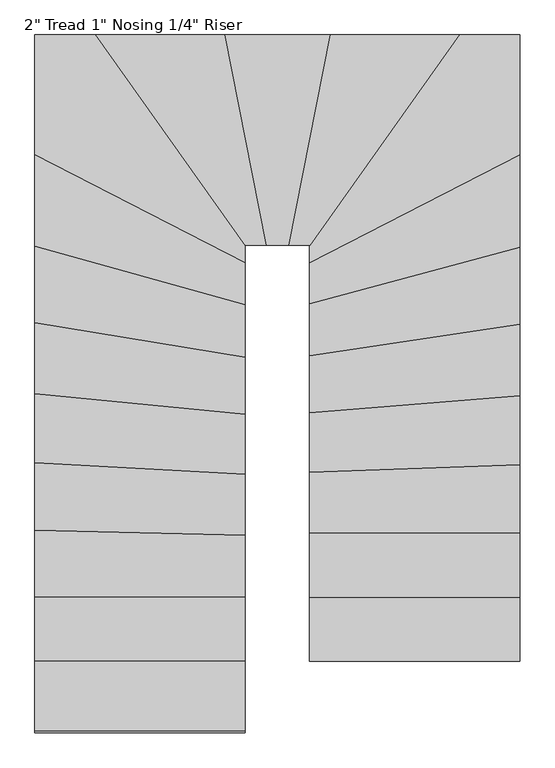
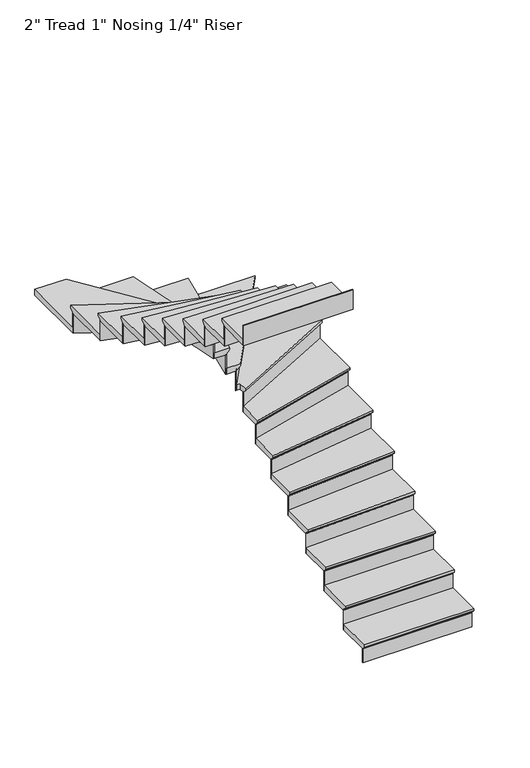
"""IFC4 building model written with IfcOpenShell, lengths in millimetres: stair flight geometry."""

from ifc_helpers import new_model, si_unit, origin, place, context, project, spatial, faceted_brep, source, transform, mapped, element, save


def stair_flight_39349fbd(model_context):
    return source(origin(), model_context, "Body", "Brep", [
        faceted_brep([(-8949.8887549, 413.7711043, 1983.9214286), (-8949.8887549, 413.7711043, 2002.9714286), (-9864.2887549, 413.7711043, 2002.9714286), (-9864.2887549, 413.7711043, 1983.9214286), (-8949.8887549, 439.1711043, 1958.5214286), (-9864.2887549, 439.1711043, 1958.5214286), (-8949.8887549, 718.5711043, 2002.9714286), (-9864.2887549, 718.5711043, 2002.9714286), (-9864.2887549, 439.1711043, 1952.1714286), (-9864.2887549, 718.5711043, 1952.1714286), (-8949.8887549, 718.5711043, 1952.1714286), (-8949.8887549, 439.1711043, 1952.1714286)], [[[0, 1, 2, 3]], [[4, 0, 3, 5]], [[2, 1, 6, 7]], [[8, 9, 10, 11]], [[2, 7, 9, 8, 5, 3]], [[8, 11, 4, 5]], [[6, 1, 0, 4, 11, 10]], [[7, 6, 10, 9]]]),
        faceted_brep([(-8949.8887549, 439.1711043, 1952.1714286), (-8949.8887549, 439.1711043, 1828.8), (-8949.8887549, 445.5211043, 1828.8), (-8949.8887549, 445.5211043, 1952.1714286), (-9864.2887549, 439.1711043, 1952.1714286), (-9864.2887549, 445.5211043, 1952.1714286), (-9864.2887549, 445.5211043, 1828.8), (-9864.2887549, 439.1711043, 1828.8)], [[[0, 1, 2, 3]], [[4, 5, 6, 7]], [[1, 0, 4, 7]], [[2, 1, 7, 6]], [[3, 2, 6, 5]], [[0, 3, 5, 4]]]),
        faceted_brep([(-8949.8887549, 718.5711043, 2126.3428571), (-8949.8887549, 718.5711043, 1952.1714286), (-8949.8887549, 724.9211043, 1952.1714286), (-8949.8887549, 724.9211043, 2126.3428571), (-9864.2887549, 718.5711043, 2126.3428571), (-9864.2887549, 724.9211043, 2126.3428571), (-9864.2887549, 724.9211043, 1952.1714286), (-9864.2887549, 718.5711043, 1952.1714286)], [[[0, 1, 2, 3]], [[4, 5, 6, 7]], [[1, 0, 4, 7]], [[2, 1, 7, 6]], [[3, 2, 6, 5]], [[0, 3, 5, 4]]]),
        faceted_brep([(-9864.2887549, 693.1711043, 2177.1428571), (-8949.8887549, 693.1711043, 2177.1428571), (-8949.8887549, 997.9711043, 2177.1428571), (-9864.2887549, 997.9711043, 2177.1428571), (-9864.2887549, 718.5711043, 2126.3428571), (-9864.2887549, 997.9711043, 2126.3428571), (-8949.8887549, 997.9711043, 2126.3428571), (-8949.8887549, 718.5711043, 2126.3428571), (-9864.2887549, 718.5711043, 2132.6928571), (-9864.2887549, 693.1711043, 2158.0928571), (-8949.8887549, 718.5711043, 2132.6928571), (-8949.8887549, 693.1711043, 2158.0928571)], [[[0, 1, 2, 3]], [[4, 5, 6, 7]], [[0, 3, 5, 4, 8, 9]], [[4, 7, 10, 8]], [[2, 1, 11, 10, 7, 6]], [[3, 2, 6, 5]], [[11, 1, 0, 9]], [[10, 11, 9, 8]]]),
        faceted_brep([(-8949.8887549, 997.9711043, 2300.5142857), (-8949.8887549, 997.9711043, 2126.3428571), (-8949.8887549, 1004.3211043, 2126.3428571), (-8949.8887549, 1004.3211043, 2300.5142857), (-9864.2887549, 997.9711043, 2300.5142857), (-9864.2887549, 1004.3211043, 2300.5142857), (-9864.2887549, 1004.3211043, 2126.3428571), (-9864.2887549, 997.9711043, 2126.3428571)], [[[0, 1, 2, 3]], [[4, 5, 6, 7]], [[1, 0, 4, 7]], [[2, 1, 7, 6]], [[3, 2, 6, 5]], [[0, 3, 5, 4]]]),
        faceted_brep([(-9864.2887549, 972.5711043, 2351.3142857), (-8949.8887549, 972.5711043, 2351.3142857), (-8949.8887549, 1292.6613973, 2351.3142857), (-9864.2887549, 1262.1091596, 2351.3142857), (-9864.2887549, 997.9711043, 2300.5142857), (-9864.2887549, 1262.1091596, 2300.5142857), (-8949.8887549, 1292.6613973, 2300.5142857), (-8949.8887549, 997.9711043, 2300.5142857), (-9864.2887549, 997.9711043, 2306.8642857), (-9864.2887549, 972.5711043, 2332.2642857), (-8949.8887549, 997.9711043, 2306.8642857), (-8949.8887549, 972.5711043, 2332.2642857)], [[[0, 1, 2, 3]], [[4, 5, 6, 7]], [[0, 3, 5, 4, 8, 9]], [[4, 7, 10, 8]], [[2, 1, 11, 10, 7, 6]], [[3, 2, 6, 5]], [[11, 1, 0, 9]], [[10, 11, 9, 8]]]),
        faceted_brep([(-8949.8887549, 1292.6613973, 2474.6857143), (-8949.8887549, 1292.6613973, 2300.5142857), (-8949.8887549, 1299.0149408, 2300.5142857), (-8949.8887549, 1299.0149408, 2474.6857143), (-9864.2887549, 1262.1091596, 2474.6857143), (-9864.2887549, 1268.4627031, 2474.6857143), (-9864.2887549, 1268.4627031, 2300.5142857), (-9864.2887549, 1262.1091596, 2300.5142857)], [[[0, 1, 2, 3]], [[4, 5, 6, 7]], [[1, 0, 4, 7]], [[2, 1, 7, 6]], [[3, 2, 6, 5]], [[0, 3, 5, 4]]]),
        faceted_brep([(-9864.2887549, 1236.6949855, 2525.4857143), (-8949.8887549, 1267.2472231, 2525.4857143), (-8949.8887549, 1593.5686288, 2525.4857143), (-9864.2887549, 1520.1371213, 2525.4857143), (-9864.2887549, 1262.1091596, 2474.6857143), (-9864.2887549, 1520.1371213, 2474.6857143), (-8949.8887549, 1593.5686288, 2474.6857143), (-8949.8887549, 1292.6613973, 2474.6857143), (-9864.2887549, 1262.1091596, 2481.0357143), (-9864.2887549, 1236.6949855, 2506.4357143), (-8949.8887549, 1292.6613973, 2481.0357143), (-8949.8887549, 1267.2472231, 2506.4357143)], [[[0, 1, 2, 3]], [[4, 5, 6, 7]], [[0, 3, 5, 4, 8, 9]], [[4, 7, 10, 8]], [[2, 1, 11, 10, 7, 6]], [[3, 2, 6, 5]], [[11, 1, 0, 9]], [[10, 11, 9, 8]]]),
        faceted_brep([(-8949.8887549, 1593.5686288, 2648.8571429), (-8949.8887549, 1593.5686288, 2474.6857143), (-8949.8887549, 1599.9390714, 2474.6857143), (-8949.8887549, 1599.9390714, 2648.8571429), (-9864.2887549, 1520.1371213, 2648.8571429), (-9864.2887549, 1526.5075639, 2648.8571429), (-9864.2887549, 1526.5075639, 2474.6857143), (-9864.2887549, 1520.1371213, 2474.6857143)], [[[0, 1, 2, 3]], [[4, 5, 6, 7]], [[1, 0, 4, 7]], [[2, 1, 7, 6]], [[3, 2, 6, 5]], [[0, 3, 5, 4]]]),
        faceted_brep([(-9864.2887549, 1494.6553506, 2699.6571429), (-8949.8887549, 1568.0868581, 2699.6571429), (-8949.8887549, 1905.4505037, 2699.6571429), (-9864.2887549, 1767.4668339, 2699.6571429), (-9864.2887549, 1520.1371213, 2648.8571429), (-9864.2887549, 1767.4668339, 2648.8571429), (-8949.8887549, 1905.4505037, 2648.8571429), (-8949.8887549, 1593.5686288, 2648.8571429), (-9864.2887549, 1520.1371213, 2655.2071429), (-9864.2887549, 1494.6553506, 2680.6071429), (-8949.8887549, 1593.5686288, 2655.2071429), (-8949.8887549, 1568.0868581, 2680.6071429)], [[[0, 1, 2, 3]], [[4, 5, 6, 7]], [[0, 3, 5, 4, 8, 9]], [[4, 7, 10, 8]], [[2, 1, 11, 10, 7, 6]], [[3, 2, 6, 5]], [[11, 1, 0, 9]], [[10, 11, 9, 8]]]),
        faceted_brep([(-8949.8887549, 1905.4505037, 2823.0285714), (-8949.8887549, 1905.4505037, 2648.8571429), (-8949.8887549, 1911.8723948, 2648.8571429), (-8949.8887549, 1911.8723948, 2823.0285714), (-9864.2887549, 1767.4668339, 2823.0285714), (-9864.2887549, 1773.888725, 2823.0285714), (-9864.2887549, 1773.888725, 2648.8571429), (-9864.2887549, 1767.4668339, 2648.8571429)], [[[0, 1, 2, 3]], [[4, 5, 6, 7]], [[1, 0, 4, 7]], [[2, 1, 7, 6]], [[3, 2, 6, 5]], [[0, 3, 5, 4]]]),
        faceted_brep([(-9864.2887549, 1741.7792694, 2873.8285714), (-8949.8887549, 1879.7629392, 2873.8285714), (-8949.8887549, 2239.5742313, 2873.8285714), (-9864.2887549, 1993.3770762, 2873.8285714), (-9864.2887549, 1767.4668339, 2823.0285714), (-9864.2887549, 1993.3770762, 2823.0285714), (-8949.8887549, 2239.5742313, 2823.0285714), (-8949.8887549, 1905.4505037, 2823.0285714), (-9864.2887549, 1767.4668339, 2829.3785714), (-9864.2887549, 1741.7792694, 2854.7785714), (-8949.8887549, 1905.4505037, 2829.3785714), (-8949.8887549, 1879.7629392, 2854.7785714)], [[[0, 1, 2, 3]], [[4, 5, 6, 7]], [[0, 3, 5, 4, 8, 9]], [[4, 7, 10, 8]], [[2, 1, 11, 10, 7, 6]], [[3, 2, 6, 5]], [[11, 1, 0, 9]], [[10, 11, 9, 8]]]),
        faceted_brep([(-8949.8887549, 2239.5742313, 2997.2), (-8949.8887549, 2239.5742313, 2823.0285714), (-8949.8887549, 2246.1503686, 2823.0285714), (-8949.8887549, 2246.1503686, 2997.2), (-9864.2887549, 1993.3770762, 2997.2), (-9864.2887549, 1999.9532136, 2997.2), (-9864.2887549, 1999.9532136, 2823.0285714), (-9864.2887549, 1993.3770762, 2823.0285714)], [[[0, 1, 2, 3]], [[4, 5, 6, 7]], [[1, 0, 4, 7]], [[2, 1, 7, 6]], [[3, 2, 6, 5]], [[0, 3, 5, 4]]]),
        faceted_brep([(-9864.2887549, 1967.0725268, 3048.0), (-8949.8887549, 2213.2696818, 3048.0), (-8949.8887549, 2644.0034455, 3048.0), (-9864.2887549, 2175.1788242, 3048.0), (-9864.2887549, 1993.3770762, 2997.2), (-9864.2887549, 2175.1788242, 2997.2), (-8949.8887549, 2644.0034455, 2997.2), (-8949.8887549, 2239.5742313, 2997.2), (-9864.2887549, 1993.3770762, 3003.55), (-9864.2887549, 1967.0725268, 3028.95), (-8949.8887549, 2239.5742313, 3003.55), (-8949.8887549, 2213.2696818, 3028.95)], [[[0, 1, 2, 3]], [[4, 5, 6, 7]], [[0, 3, 5, 4, 8, 9]], [[4, 7, 10, 8]], [[2, 1, 11, 10, 7, 6]], [[3, 2, 6, 5]], [[11, 1, 0, 9]], [[10, 11, 9, 8]]]),
        faceted_brep([(-8949.8887549, 2644.0034455, 3171.3714286), (-8949.8887549, 2644.0034455, 2997.2), (-8949.8887549, 2651.1394286, 2997.2), (-8949.8887549, 2651.1394286, 3171.3714286), (-9864.2887549, 2175.1788242, 3171.3714286), (-9864.2887549, 2182.3148073, 3171.3714286), (-9864.2887549, 2182.3148073, 2997.2), (-9864.2887549, 2175.1788242, 2997.2)], [[[0, 1, 2, 3]], [[4, 5, 6, 7]], [[1, 0, 4, 7]], [[2, 1, 7, 6]], [[3, 2, 6, 5]], [[0, 3, 5, 4]]]),
        faceted_brep([(-9893.8438377, 2220.9027962, 3222.1714286), (-9864.2887549, 2220.9027962, 3222.1714286), (-9864.2887549, 2146.6348916, 3222.1714286), (-8949.8887549, 2615.459513, 3222.1714286), (-8949.8887549, 3135.3027962, 3222.1714286), (-9243.5698886, 3135.3027962, 3222.1714286), (-9864.2887549, 2220.9027962, 3171.3714286), (-9893.8438377, 2220.9027962, 3171.3714286), (-9243.5698886, 3135.3027962, 3171.3714286), (-8949.8887549, 3135.3027962, 3171.3714286), (-8949.8887549, 2644.0034455, 3171.3714286), (-9864.2887549, 2175.1788242, 3171.3714286), (-8949.8887549, 2644.0034455, 3177.7214286), (-9864.2887549, 2175.1788242, 3177.7214286), (-8949.8887549, 2615.459513, 3203.1214286), (-9864.2887549, 2146.6348916, 3203.1214286)], [[[0, 1, 2, 3, 4, 5]], [[6, 7, 8, 9, 10, 11]], [[1, 0, 7, 6]], [[11, 10, 12, 13]], [[4, 3, 14, 12, 10, 9]], [[0, 5, 8, 7]], [[14, 3, 2, 15]], [[12, 14, 15, 13]], [[2, 1, 6, 11, 13, 15]], [[5, 4, 9, 8]]]),
        faceted_brep([(-9243.5698886, 3135.3027962, 3345.5428571), (-9243.5698886, 3135.3027962, 3171.3714286), (-9251.3618634, 3135.3027962, 3171.3714286), (-9251.3618634, 3135.3027962, 3345.5428571), (-9893.8438377, 2220.9027962, 3345.5428571), (-9901.6358125, 2220.9027962, 3345.5428571), (-9901.6358125, 2220.9027962, 3171.3714286), (-9893.8438377, 2220.9027962, 3171.3714286)], [[[0, 1, 2, 3]], [[4, 5, 6, 7]], [[1, 0, 4, 7]], [[2, 1, 7, 6]], [[3, 2, 6, 5]], [[0, 3, 5, 4]]]),
        faceted_brep([(-9862.6759385, 2220.9027962, 3396.3428571), (-9212.4019894, 3135.3027962, 3396.3428571), (-9800.0570685, 3135.3027962, 3396.3428571), (-9980.2979248, 2220.9027962, 3396.3428571), (-9893.8438377, 2220.9027962, 3345.5428571), (-9980.2979248, 2220.9027962, 3345.5428571), (-9800.0570685, 3135.3027962, 3345.5428571), (-9243.5698886, 3135.3027962, 3345.5428571), (-9893.8438377, 2220.9027962, 3351.8928571), (-9862.6759385, 2220.9027962, 3377.2928571), (-9243.5698886, 3135.3027962, 3351.8928571), (-9212.4019894, 3135.3027962, 3377.2928571)], [[[0, 1, 2, 3]], [[4, 5, 6, 7]], [[0, 3, 5, 4, 8, 9]], [[4, 7, 10, 8]], [[2, 1, 11, 10, 7, 6]], [[3, 2, 6, 5]], [[11, 1, 0, 9]], [[10, 11, 9, 8]]]),
        faceted_brep([(-9800.0570685, 3135.3027962, 3519.7142857), (-9800.0570685, 3135.3027962, 3345.5428571), (-9806.5292539, 3135.3027962, 3345.5428571), (-9806.5292539, 3135.3027962, 3519.7142857), (-9980.2979248, 2220.9027962, 3519.7142857), (-9986.7701102, 2220.9027962, 3519.7142857), (-9986.7701102, 2220.9027962, 3345.5428571), (-9980.2979248, 2220.9027962, 3345.5428571)], [[[0, 1, 2, 3]], [[4, 5, 6, 7]], [[1, 0, 4, 7]], [[2, 1, 7, 6]], [[3, 2, 6, 5]], [[0, 3, 5, 4]]]),
        faceted_brep([(-9954.409183, 2220.9027962, 3570.5142857), (-9774.1683267, 3135.3027962, 3570.5142857), (-10259.6979248, 3135.3027962, 3570.5142857), (-10079.4570685, 2220.9027962, 3570.5142857), (-9980.2979248, 2220.9027962, 3519.7142857), (-10079.4570685, 2220.9027962, 3519.7142857), (-10259.6979248, 3135.3027962, 3519.7142857), (-9800.0570685, 3135.3027962, 3519.7142857), (-9980.2979248, 2220.9027962, 3526.0642857), (-9954.409183, 2220.9027962, 3551.4642857), (-9800.0570685, 3135.3027962, 3526.0642857), (-9774.1683267, 3135.3027962, 3551.4642857)], [[[0, 1, 2, 3]], [[4, 5, 6, 7]], [[0, 3, 5, 4, 8, 9]], [[4, 7, 10, 8]], [[3, 2, 6, 5]], [[11, 1, 0, 9]], [[10, 11, 9, 8]], [[2, 1, 11, 10, 7, 6]]]),
        faceted_brep([(-10259.6979248, 3135.3027962, 3693.8857143), (-10259.6979248, 3135.3027962, 3519.7142857), (-10266.1701102, 3135.3027962, 3519.7142857), (-10266.1701102, 3135.3027962, 3693.8857143), (-10079.4570685, 2220.9027962, 3693.8857143), (-10085.9292539, 2220.9027962, 3693.8857143), (-10085.9292539, 2220.9027962, 3519.7142857), (-10079.4570685, 2220.9027962, 3519.7142857)], [[[0, 1, 2, 3]], [[4, 5, 6, 7]], [[1, 0, 4, 7]], [[2, 1, 7, 6]], [[3, 2, 6, 5]], [[0, 3, 5, 4]]]),
        faceted_brep([(-10143.6887549, 2174.8073217, 3744.6857143), (-10143.6887549, 2220.9027962, 3744.6857143), (-10053.5683267, 2220.9027962, 3744.6857143), (-10233.809183, 3135.3027962, 3744.6857143), (-10826.7434195, 3135.3027962, 3744.6857143), (-10143.6887549, 2220.9027962, 3693.8857143), (-10143.6887549, 2174.8073217, 3693.8857143), (-10826.7434195, 3135.3027962, 3693.8857143), (-10259.6979248, 3135.3027962, 3693.8857143), (-10079.4570685, 2220.9027962, 3693.8857143), (-10259.6979248, 3135.3027962, 3700.2357143), (-10079.4570685, 2220.9027962, 3700.2357143), (-10233.809183, 3135.3027962, 3725.6357143), (-10053.5683267, 2220.9027962, 3725.6357143)], [[[0, 1, 2, 3, 4]], [[5, 6, 7, 8, 9]], [[1, 0, 6, 5]], [[9, 8, 10, 11]], [[4, 3, 12, 10, 8, 7]], [[0, 4, 7, 6]], [[12, 3, 2, 13]], [[10, 12, 13, 11]], [[2, 1, 5, 9, 11, 13]]]),
        faceted_brep([(-10826.7434195, 3135.3027962, 3868.0571429), (-10826.7434195, 3135.3027962, 3693.8857143), (-10834.5353943, 3135.3027962, 3693.8857143), (-10834.5353943, 3135.3027962, 3868.0571429), (-10143.6887549, 2174.8073217, 3868.0571429), (-10143.6887549, 2163.8504292, 3868.0571429), (-10143.6887549, 2163.8504292, 3693.8857143), (-10143.6887549, 2174.8073217, 3693.8857143)], [[[0, 1, 2, 3]], [[4, 5, 6, 7]], [[1, 0, 4, 7]], [[2, 1, 7, 6]], [[3, 2, 6, 5]], [[0, 3, 5, 4]]]),
        faceted_brep([(-10143.6887549, 2218.6348916, 3918.8571429), (-10795.5755204, 3135.3027962, 3918.8571429), (-11058.0887549, 3135.3027962, 3918.8571429), (-11058.0887549, 2586.9155804, 3918.8571429), (-10143.6887549, 2118.0909591, 3918.8571429), (-10143.6887549, 2174.8073217, 3868.0571429), (-10143.6887549, 2118.0909591, 3868.0571429), (-11058.0887549, 2586.9155804, 3868.0571429), (-11058.0887549, 3135.3027962, 3868.0571429), (-10826.7434195, 3135.3027962, 3868.0571429), (-10143.6887549, 2174.8073217, 3874.4071429), (-10143.6887549, 2218.6348916, 3899.8071429), (-10826.7434195, 3135.3027962, 3874.4071429), (-10795.5755204, 3135.3027962, 3899.8071429)], [[[0, 1, 2, 3, 4]], [[5, 6, 7, 8, 9]], [[0, 4, 6, 5, 10, 11]], [[5, 9, 12, 10]], [[2, 1, 13, 12, 9, 8]], [[3, 2, 8, 7]], [[4, 3, 7, 6]], [[13, 1, 0, 11]], [[12, 13, 11, 10]]]),
        faceted_brep([(-11058.0887549, 2586.9155804, 4042.2285714), (-11058.0887549, 2586.9155804, 3868.0571429), (-11058.0887549, 2579.7795973, 3868.0571429), (-11058.0887549, 2579.7795973, 4042.2285714), (-10143.6887549, 2118.0909591, 4042.2285714), (-10143.6887549, 2110.954976, 4042.2285714), (-10143.6887549, 2110.954976, 3868.0571429), (-10143.6887549, 2118.0909591, 3868.0571429)], [[[0, 1, 2, 3]], [[4, 5, 6, 7]], [[1, 0, 4, 7]], [[2, 1, 7, 6]], [[3, 2, 6, 5]], [[0, 3, 5, 4]]]),
        faceted_brep([(-10143.6887549, 2146.6348916, 4093.0285714), (-11058.0887549, 2615.459513, 4093.0285714), (-11058.0887549, 2190.4900593, 4093.0285714), (-10143.6887549, 1937.1383148, 4093.0285714), (-10143.6887549, 2118.0909591, 4042.2285714), (-10143.6887549, 1937.1383148, 4042.2285714), (-11058.0887549, 2190.4900593, 4042.2285714), (-11058.0887549, 2586.9155804, 4042.2285714), (-10143.6887549, 2118.0909591, 4048.5785714), (-10143.6887549, 2146.6348916, 4073.9785714), (-11058.0887549, 2586.9155804, 4048.5785714), (-11058.0887549, 2615.459513, 4073.9785714)], [[[0, 1, 2, 3]], [[4, 5, 6, 7]], [[0, 3, 5, 4, 8, 9]], [[4, 7, 10, 8]], [[2, 1, 11, 10, 7, 6]], [[3, 2, 6, 5]], [[11, 1, 0, 9]], [[10, 11, 9, 8]]]),
        faceted_brep([(-11058.0887549, 2190.4900593, 4216.4), (-11058.0887549, 2190.4900593, 4042.2285714), (-11058.0887549, 2183.90083, 4042.2285714), (-11058.0887549, 2183.90083, 4216.4), (-10143.6887549, 1937.1383148, 4216.4), (-10143.6887549, 1930.5490855, 4216.4), (-10143.6887549, 1930.5490855, 4042.2285714), (-10143.6887549, 1937.1383148, 4042.2285714)], [[[0, 1, 2, 3]], [[4, 5, 6, 7]], [[1, 0, 4, 7]], [[2, 1, 7, 6]], [[3, 2, 6, 5]], [[0, 3, 5, 4]]]),
        faceted_brep([(-10143.6887549, 1963.4952321, 4267.2), (-11058.0887549, 2216.8469766, 4267.2), (-11058.0887549, 1860.2592576, 4267.2), (-10143.6887549, 1709.7998423, 4267.2), (-10143.6887549, 1937.1383148, 4216.4), (-10143.6887549, 1709.7998423, 4216.4), (-11058.0887549, 1860.2592576, 4216.4), (-11058.0887549, 2190.4900593, 4216.4), (-10143.6887549, 1937.1383148, 4222.75), (-10143.6887549, 1963.4952321, 4248.15), (-11058.0887549, 2190.4900593, 4222.75), (-11058.0887549, 2216.8469766, 4248.15)], [[[0, 1, 2, 3]], [[4, 5, 6, 7]], [[0, 3, 5, 4, 8, 9]], [[4, 7, 10, 8]], [[2, 1, 11, 10, 7, 6]], [[3, 2, 6, 5]], [[11, 1, 0, 9]], [[10, 11, 9, 8]]]),
        faceted_brep([(-11058.0887549, 1860.2592576, 4390.5714286), (-11058.0887549, 1860.2592576, 4216.4), (-11058.0887549, 1853.823869, 4216.4), (-11058.0887549, 1853.823869, 4390.5714286), (-10143.6887549, 1709.7998423, 4390.5714286), (-10143.6887549, 1703.3644537, 4390.5714286), (-10143.6887549, 1703.3644537, 4216.4), (-10143.6887549, 1709.7998423, 4216.4)], [[[0, 1, 2, 3]], [[4, 5, 6, 7]], [[1, 0, 4, 7]], [[2, 1, 7, 6]], [[3, 2, 6, 5]], [[0, 3, 5, 4]]]),
        faceted_brep([(-10143.6887549, 1735.5413967, 4441.3714286), (-11058.0887549, 1886.000812, 4441.3714286), (-11058.0887549, 1550.7121779, 4441.3714286), (-10143.6887549, 1460.9860489, 4441.3714286), (-10143.6887549, 1709.7998423, 4390.5714286), (-10143.6887549, 1460.9860489, 4390.5714286), (-11058.0887549, 1550.7121779, 4390.5714286), (-11058.0887549, 1860.2592576, 4390.5714286), (-10143.6887549, 1709.7998423, 4396.9214286), (-10143.6887549, 1735.5413967, 4422.3214286), (-11058.0887549, 1860.2592576, 4396.9214286), (-11058.0887549, 1886.000812, 4422.3214286)], [[[0, 1, 2, 3]], [[4, 5, 6, 7]], [[0, 3, 5, 4, 8, 9]], [[4, 7, 10, 8]], [[2, 1, 11, 10, 7, 6]], [[3, 2, 6, 5]], [[11, 1, 0, 9]], [[10, 11, 9, 8]]]),
        faceted_brep([(-11058.0887549, 1550.7121779, 4564.7428571), (-11058.0887549, 1550.7121779, 4390.5714286), (-11058.0887549, 1544.3316802, 4390.5714286), (-11058.0887549, 1544.3316802, 4564.7428571), (-10143.6887549, 1460.9860489, 4564.7428571), (-10143.6887549, 1454.6055511, 4564.7428571), (-10143.6887549, 1454.6055511, 4390.5714286), (-10143.6887549, 1460.9860489, 4390.5714286)], [[[0, 1, 2, 3]], [[4, 5, 6, 7]], [[1, 0, 4, 7]], [[2, 1, 7, 6]], [[3, 2, 6, 5]], [[0, 3, 5, 4]]]),
        faceted_brep([(-10143.6887549, 1486.5080398, 4615.5428571), (-11058.0887549, 1576.2341688, 4615.5428571), (-11058.0887549, 1251.3568844, 4615.5428571), (-10143.6887549, 1201.7105044, 4615.5428571), (-10143.6887549, 1460.9860489, 4564.7428571), (-10143.6887549, 1201.7105044, 4564.7428571), (-11058.0887549, 1251.3568844, 4564.7428571), (-11058.0887549, 1550.7121779, 4564.7428571), (-10143.6887549, 1460.9860489, 4571.0928571), (-10143.6887549, 1486.5080398, 4596.4928571), (-11058.0887549, 1550.7121779, 4571.0928571), (-11058.0887549, 1576.2341688, 4596.4928571)], [[[0, 1, 2, 3]], [[4, 5, 6, 7]], [[0, 3, 5, 4, 8, 9]], [[4, 7, 10, 8]], [[2, 1, 11, 10, 7, 6]], [[3, 2, 6, 5]], [[11, 1, 0, 9]], [[10, 11, 9, 8]]]),
        faceted_brep([(-11058.0887549, 1251.3568844, 4738.9142857), (-11058.0887549, 1251.3568844, 4564.7428571), (-11058.0887549, 1244.9975319, 4564.7428571), (-11058.0887549, 1244.9975319, 4738.9142857), (-10143.6887549, 1201.7105044, 4738.9142857), (-10143.6887549, 1195.3511519, 4738.9142857), (-10143.6887549, 1195.3511519, 4564.7428571), (-10143.6887549, 1201.7105044, 4564.7428571)], [[[0, 1, 2, 3]], [[4, 5, 6, 7]], [[1, 0, 4, 7]], [[2, 1, 7, 6]], [[3, 2, 6, 5]], [[0, 3, 5, 4]]]),
        faceted_brep([(-10143.6887549, 1227.1479143, 4789.7142857), (-11058.0887549, 1276.7942943, 4789.7142857), (-11058.0887549, 957.7721544, 4789.7142857), (-10143.6887549, 936.5563826, 4789.7142857), (-10143.6887549, 1201.7105044, 4738.9142857), (-10143.6887549, 936.5563826, 4738.9142857), (-11058.0887549, 957.7721544, 4738.9142857), (-11058.0887549, 1251.3568844, 4738.9142857), (-10143.6887549, 1201.7105044, 4745.2642857), (-10143.6887549, 1227.1479143, 4770.6642857), (-11058.0887549, 1251.3568844, 4745.2642857), (-11058.0887549, 1276.7942943, 4770.6642857)], [[[0, 1, 2, 3]], [[4, 5, 6, 7]], [[0, 3, 5, 4, 8, 9]], [[4, 7, 10, 8]], [[2, 1, 11, 10, 7, 6]], [[3, 2, 6, 5]], [[11, 1, 0, 9]], [[10, 11, 9, 8]]]),
        faceted_brep([(-11058.0887549, 957.7721544, 4913.0857143), (-11058.0887549, 957.7721544, 4738.9142857), (-11058.0887549, 951.4204454, 4738.9142857), (-11058.0887549, 951.4204454, 4913.0857143), (-10143.6887549, 936.5563826, 4913.0857143), (-10143.6887549, 930.2046737, 4913.0857143), (-10143.6887549, 930.2046737, 4738.9142857), (-10143.6887549, 936.5563826, 4738.9142857)], [[[0, 1, 2, 3]], [[4, 5, 6, 7]], [[1, 0, 4, 7]], [[2, 1, 7, 6]], [[3, 2, 6, 5]], [[0, 3, 5, 4]]]),
        faceted_brep([(-10143.6887549, 961.9632184, 4963.8857143), (-11058.0887549, 983.1789902, 4963.8857143), (-11058.0887549, 667.7711043, 4963.8857143), (-10143.6887549, 667.7711043, 4963.8857143), (-10143.6887549, 936.5563826, 4913.0857143), (-10143.6887549, 667.7711043, 4913.0857143), (-11058.0887549, 667.7711043, 4913.0857143), (-11058.0887549, 957.7721544, 4913.0857143), (-10143.6887549, 936.5563826, 4919.4357143), (-10143.6887549, 961.9632184, 4944.8357143), (-11058.0887549, 957.7721544, 4919.4357143), (-11058.0887549, 983.1789902, 4944.8357143)], [[[0, 1, 2, 3]], [[4, 5, 6, 7]], [[0, 3, 5, 4, 8, 9]], [[4, 7, 10, 8]], [[2, 1, 11, 10, 7, 6]], [[3, 2, 6, 5]], [[11, 1, 0, 9]], [[10, 11, 9, 8]]]),
        faceted_brep([(-11058.0887549, 667.7711043, 5087.2571429), (-11058.0887549, 667.7711043, 4913.0857143), (-11058.0887549, 661.4211043, 4913.0857143), (-11058.0887549, 661.4211043, 5087.2571429), (-10143.6887549, 667.7711043, 5087.2571429), (-10143.6887549, 661.4211043, 5087.2571429), (-10143.6887549, 661.4211043, 4913.0857143), (-10143.6887549, 667.7711043, 4913.0857143)], [[[0, 1, 2, 3]], [[4, 5, 6, 7]], [[1, 0, 4, 7]], [[2, 1, 7, 6]], [[3, 2, 6, 5]], [[0, 3, 5, 4]]]),
        faceted_brep([(-10143.6887549, 693.1711043, 5138.0571429), (-11058.0887549, 693.1711043, 5138.0571429), (-11058.0887549, 388.3711043, 5138.0571429), (-10143.6887549, 388.3711043, 5138.0571429), (-10143.6887549, 667.7711043, 5087.2571429), (-10143.6887549, 388.3711043, 5087.2571429), (-11058.0887549, 388.3711043, 5087.2571429), (-11058.0887549, 667.7711043, 5087.2571429), (-10143.6887549, 667.7711043, 5093.6071429), (-10143.6887549, 693.1711043, 5119.0071429), (-11058.0887549, 667.7711043, 5093.6071429), (-11058.0887549, 693.1711043, 5119.0071429)], [[[0, 1, 2, 3]], [[4, 5, 6, 7]], [[0, 3, 5, 4, 8, 9]], [[4, 7, 10, 8]], [[2, 1, 11, 10, 7, 6]], [[3, 2, 6, 5]], [[11, 1, 0, 9]], [[10, 11, 9, 8]]]),
        faceted_brep([(-11058.0887549, 388.3711043, 5261.4285714), (-11058.0887549, 388.3711043, 5087.2571429), (-11058.0887549, 382.0211043, 5087.2571429), (-11058.0887549, 382.0211043, 5261.4285714), (-10143.6887549, 388.3711043, 5261.4285714), (-10143.6887549, 382.0211043, 5261.4285714), (-10143.6887549, 382.0211043, 5087.2571429), (-10143.6887549, 388.3711043, 5087.2571429)], [[[0, 1, 2, 3]], [[4, 5, 6, 7]], [[1, 0, 4, 7]], [[2, 1, 7, 6]], [[3, 2, 6, 5]], [[0, 3, 5, 4]]]),
        faceted_brep([(-11058.0887549, 108.9711043, 5435.6), (-11058.0887549, 108.9711043, 5261.4285714), (-11058.0887549, 102.6211043, 5261.4285714), (-11058.0887549, 102.6211043, 5435.6), (-10143.6887549, 108.9711043, 5435.6), (-10143.6887549, 102.6211043, 5435.6), (-10143.6887549, 102.6211043, 5261.4285714), (-10143.6887549, 108.9711043, 5261.4285714)], [[[0, 1, 2, 3]], [[4, 5, 6, 7]], [[1, 0, 4, 7]], [[2, 1, 7, 6]], [[3, 2, 6, 5]], [[0, 3, 5, 4]]]),
        faceted_brep([(-10143.6887549, 413.7711043, 5312.2285714), (-11058.0887549, 413.7711043, 5312.2285714), (-11058.0887549, 108.9711043, 5312.2285714), (-10143.6887549, 108.9711043, 5312.2285714), (-10143.6887549, 388.3711043, 5261.4285714), (-10143.6887549, 108.9711043, 5261.4285714), (-11058.0887549, 108.9711043, 5261.4285714), (-11058.0887549, 388.3711043, 5261.4285714), (-10143.6887549, 388.3711043, 5267.7785714), (-10143.6887549, 413.7711043, 5293.1785714), (-11058.0887549, 388.3711043, 5267.7785714), (-11058.0887549, 413.7711043, 5293.1785714)], [[[0, 1, 2, 3]], [[4, 5, 6, 7]], [[0, 3, 5, 4, 8, 9]], [[4, 7, 10, 8]], [[2, 1, 11, 10, 7, 6]], [[3, 2, 6, 5]], [[11, 1, 0, 9]], [[10, 11, 9, 8]]]),
    ])


if __name__ == "__main__":
    model = new_model("IFC4")
    model_context = context("Model", 3, world=origin())
    ifc_project = project(units=[si_unit("LENGTHUNIT", "METRE", prefix="MILLI")], contexts=[model_context])
    site = spatial("IfcSite", under=ifc_project)
    building = spatial("IfcBuilding", under=site)
    placement = place(None, origin())
    stair_flight_shape = stair_flight_39349fbd(model_context)
    element("IfcStairFlight", 1, ObjectType="2\" Tread 1\" Nosing 1/4\" Riser", at=placement, inside=building, context=model_context, shape_type="MappedRepresentation", body=[
        mapped(stair_flight_shape, transform((0.0, 0.0, 0.0), x_axis=(1.0, 0.0, 0.0), y_axis=(0.0, 1.0, 0.0), z_axis=(0.0, 0.0, 1.0))),
    ])
    save(model, "model.ifc")
